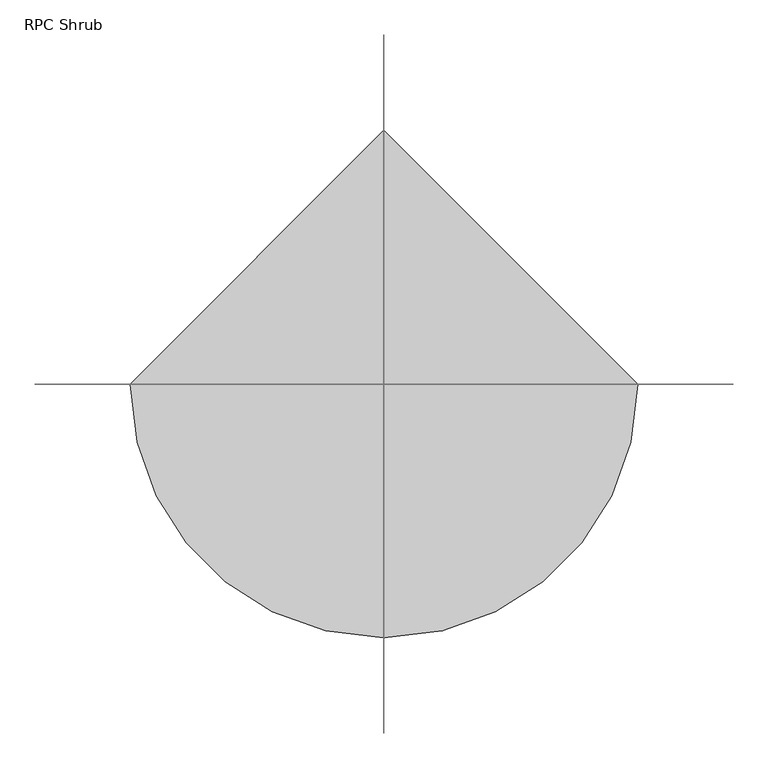
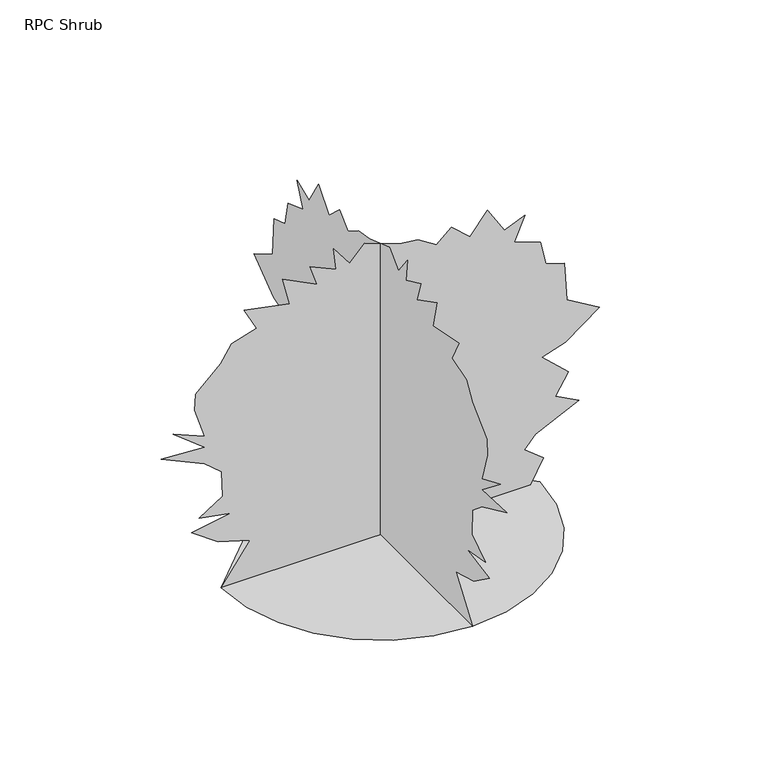
"""IFC4 building model written with IfcOpenShell, lengths in millimetres: geographic element geometry, RPC Shrub."""

from ifc_helpers import new_model, si_unit, origin, place, context, project, spatial, triangles, source, transform, mapped, element, save


def rpc_shrub_d2795376(model_context):
    return source(origin(), model_context, "Body", "Tessellation", [
        triangles([(-812.5409557, 0.0, 3.62e-05), (-791.0601448, -186.180478, 3.62e-05), (-729.8816843, -357.1570149, 3.62e-05), (-633.9078186, -508.0330164, 3.62e-05), (-508.0330164, -633.9078186, 3.62e-05), (-357.1570149, -729.8816843, 3.62e-05), (-186.180478, -791.0601448, 3.62e-05), (3.55e-05, -812.5409557, 3.62e-05), (186.180478, -791.0601448, 3.62e-05), (357.1570149, -729.8816843, 3.62e-05), (508.0330164, -633.9078186, 3.62e-05), (633.9078186, -508.0330164, 3.62e-05), (729.8816843, -357.1570149, 3.62e-05), (791.0601448, -186.180478, 3.62e-05), (812.5409557, 7.1e-05, 3.62e-05), (-0.0001066, 812.5409557, 3.62e-05), (-0.0042747, -811.2988804, 0.0001209), (-0.0042708, -665.7314575, 204.5081021), (-0.004267, -827.9002653, 251.4511125), (-0.004262, -964.4608252, 349.6055863), (-0.004264, -763.884696, 383.7457263), (-0.0042607, -926.0535038, 413.6186849), (-0.0042602, -806.5617422, 490.4333639), (-0.0042562, -810.8289963, 622.7267424), (-0.0042527, -896.1805452, 695.2767471), (-0.0042464, -1118.0927267, 797.697167), (-0.0042501, -896.1805452, 784.8930067), (-0.0042438, -1058.3468822, 912.9192038), (-0.0042483, -896.1805452, 844.6389238), (-0.0042428, -947.3895561, 1002.5380068), (-0.0042404, -943.1223021, 1087.8896284), (-0.0042387, -815.0961777, 1207.38139), (-0.0042368, -759.6175146, 1297.000193), (-0.0042376, -631.5913176, 1335.4075871), (-0.0042331, -695.6044161, 1454.899276), (-0.0042379, -465.1578355, 1407.9550484), (-0.0042331, -499.2979754, 1553.0525871), (-0.0042384, -324.3300579, 1463.4336388), (-0.0042347, -358.4701979, 1570.1213127), (-0.0042384, -226.1755659, 1510.3753956), (-0.0042348, -238.9781819, 1625.6000484), (-0.0042392, -157.8947773, 1518.9123745), (-0.0042379, -81.0790899, 1599.9941986), (-0.0042425, 98.1577894, 1535.9812454), (-0.0042443, 192.0433106, 1523.1795559), (-0.0042475, 285.9303487, 1463.4336388), (-0.0042466, 362.7450096, 1531.7139187), (-0.0042505, 456.6310304, 1446.3622971), (-0.0042486, 546.2498697, 1557.3197685), (-0.0042539, 631.6014914, 1420.7592087), (-0.0042542, 738.2890926, 1463.4336388), (-0.0042571, 682.8104296, 1339.6747684), (-0.0042604, 815.1063515, 1292.7303955), (-0.0042647, 844.9766939, 1164.7042711), (-0.004267, 938.862751, 1134.8313852), (-0.0042731, 951.6669113, 934.2577269), (-0.0042786, 1118.1003571, 836.1044884), (-0.0042798, 943.1324759, 708.078364), (-0.0042791, 823.6407143, 669.67097), (-0.004285, 960.2012741, 541.6448456), (-0.0042871, 891.9209942, 434.9546645), (-0.0042908, 1011.4127558, 370.9416023), (-0.0042907, 789.5005743, 264.2539829), (-0.0042918, 734.0219112, 200.2406482), (-0.0042955, 832.1751497, 123.4246974), (-0.0042982, 766.4170269, 0.0205859), (-811.3090542, 0.0043453, 0.0), (-665.7416313, 0.0043331, 204.5081021), (-827.9078957, 0.0043303, 251.4511125), (-964.4684555, 0.0043245, 349.6055863), (-763.8948698, 0.0043224, 383.7457263), (-926.0611341, 0.0043206, 413.6186849), (-806.5693726, 0.0043161, 490.4333639), (-810.836554, 0.0043082, 622.7267424), (-896.1881756, 0.0043039, 695.2742037), (-1118.1003571, 0.0042978, 797.697167), (-896.1881756, 0.0042985, 784.8930067), (-1058.3545126, 0.0042909, 912.9192038), (-896.1881756, 0.004295, 844.6389238), (-947.3996572, 0.0042855, 1002.5380068), (-943.1299324, 0.0042805, 1087.8896284), (-815.1063515, 0.0042733, 1207.38139), (-759.6276157, 0.004268, 1297.000193), (-631.6014914, 0.0042657, 1335.4075871), (-695.6145899, 0.0042586, 1454.899276), (-465.1654295, 0.0042614, 1407.9550484), (-499.3055695, 0.0042527, 1553.0525871), (-324.3376883, 0.0042581, 1463.4336388), (-358.4778282, 0.0042517, 1570.1213127), (-226.1839592, 0.0042553, 1510.3753956), (-238.9868297, 0.0042484, 1625.6000484), (-157.903425, 0.0042548, 1518.9123745), (-81.0877195, 0.0042499, 1599.9941986), (98.1491599, 0.0042537, 1535.9812454), (192.0346629, 0.0042545, 1523.1795559), (285.9201749, 0.0042581, 1463.4336388), (362.7374156, 0.004254, 1531.7139187), (456.6234364, 0.0042591, 1446.3622971), (546.2422394, 0.0042525, 1557.3197685), (631.5913176, 0.0042606, 1420.7565926), (738.2814623, 0.0042581, 1463.4336388), (682.8027992, 0.0042654, 1339.6747684), (815.0961777, 0.0042682, 1292.7303955), (844.9691362, 0.0042759, 1164.7042711), (938.8551207, 0.0042777, 1134.8313852), (951.6567375, 0.0042896, 934.2577269), (1118.0927267, 0.0042955, 836.1044884), (943.1223021, 0.0043031, 708.078364), (823.6305405, 0.0043054, 669.67097), (960.1936438, 0.004313, 541.6448456), (891.9133638, 0.0043194, 434.9546645), (1011.402582, 0.0043232, 370.9416023), (789.4904005, 0.0043296, 264.2539829), (734.0142809, 0.0043334, 200.2403938), (832.1675194, 0.0043379, 123.4246974), (766.4094692, 0.0043453, 0.020512)], [[15, 16, 1], [14, 15, 1], [14, 1, 2], [13, 14, 2], [13, 2, 3], [13, 3, 4], [12, 13, 4], [11, 12, 4], [11, 4, 5], [11, 5, 6], [11, 6, 7], [11, 7, 8], [11, 8, 9], [11, 9, 10], [27, 28, 29], [25, 26, 27], [40, 41, 42], [21, 22, 23], [50, 51, 52], [19, 20, 21], [38, 39, 40], [36, 37, 38], [34, 35, 36], [61, 62, 63], [66, 17, 18], [56, 57, 58], [48, 49, 50], [18, 19, 21], [46, 47, 48], [64, 65, 66], [59, 60, 61], [56, 58, 59], [54, 55, 56], [42, 43, 44], [52, 53, 54], [54, 56, 59], [24, 25, 27], [48, 50, 52], [59, 61, 63], [52, 54, 59], [48, 52, 59], [46, 48, 59], [66, 18, 21], [30, 31, 32], [29, 30, 32], [66, 21, 23], [66, 23, 24], [64, 66, 24], [63, 64, 24], [59, 63, 24], [46, 59, 24], [45, 46, 24], [44, 45, 24], [42, 44, 24], [40, 42, 24], [38, 40, 24], [36, 38, 24], [34, 36, 24], [34, 24, 27], [34, 27, 29], [34, 29, 32], [33, 34, 32], [77, 78, 79], [75, 76, 77], [90, 91, 92], [71, 72, 73], [100, 101, 102], [69, 70, 71], [88, 89, 90], [86, 87, 88], [84, 85, 86], [111, 112, 113], [116, 67, 68], [106, 107, 108], [98, 99, 100], [68, 69, 71], [96, 97, 98], [114, 115, 116], [109, 110, 111], [106, 108, 109], [104, 105, 106], [92, 93, 94], [102, 103, 104], [104, 106, 109], [74, 75, 77], [98, 100, 102], [109, 111, 113], [102, 104, 109], [98, 102, 109], [96, 98, 109], [116, 68, 71], [80, 81, 82], [79, 80, 82], [116, 71, 73], [116, 73, 74], [114, 116, 74], [113, 114, 74], [109, 113, 74], [96, 109, 74], [95, 96, 74], [94, 95, 74], [92, 94, 74], [90, 92, 74], [88, 90, 74], [86, 88, 74], [84, 86, 74], [84, 74, 77], [84, 77, 79], [84, 79, 82], [83, 84, 82]], closed=False),
    ])


if __name__ == "__main__":
    model = new_model("IFC4")
    model_context = context("Model", 3, world=origin())
    ifc_project = project(units=[si_unit("LENGTHUNIT", "METRE", prefix="MILLI")], contexts=[model_context])
    site = spatial("IfcSite", under=ifc_project)
    building = spatial("IfcBuilding", under=site)
    placement = place(None, origin())
    rpc_shrub_shape = rpc_shrub_d2795376(model_context)
    element("IfcGeographicElement", 1, ObjectType="RPC Shrub", at=placement, inside=building, context=model_context, shape_type="MappedRepresentation", body=[
        mapped(rpc_shrub_shape, transform((0.0, 0.0, 0.0), x_axis=(1.0, 0.0, 0.0), y_axis=(0.0, 1.0, 0.0), z_axis=(0.0, 0.0, 1.0))),
    ])
    save(model, "model.ifc")

# Revit data of these elements
# Type "RPC Shrub"
#   built-in parameter 1005198 = "{2, 15},{39, RPC-16-G3GJ-A6PX-PK1P-U000-ST1L-LVER-AU},{1, 0},{1, 0},{2, 35},{1, 8},{5, Color},{1, 0},{1, 0},{3, 0.8},{3, 0.8},{3, 0.8},{1, 8},{7, BBoxMin},{1, 0},{1, 0},{1, 0},{1, 0},{1, 0},{1, 8},{7, BBoxMax},{1, 0},{1, 0},{1, 0},{1, 0},{1, 0},{2, 11},{9, RPCTypeId},{1, 0},{1, 0},{39, RPC-16-G3GJ-A6PX-PK1P-U000-ST1L-LVER-AU},{1, 6},{14, RPCPlantHeight},{1, 0},{1, 0},{7, 5.33333},{2, 11},{7, keyword},{1, 0},{1, 0},{22, :Geometry:RPC:Oleander},{2, 11},{8, category},{1, 0},{1, 0},{17, :Shrubs & Grasses},{2, 11},{12, LocalizedUID},{1, 0},{1, 0},{8, Oleander},{2, 14},{6, Height},{1, 0},{1, 0},{7, 5.33333},{1, 2},{16, Cast Reflections},{1, 0},{1, 0},{1, 0},{1, 2},{12, Cast Shadows},{1, 0},{1, 0},{1, 1},{1, 2},{9, Lock View},{1, 0},{1, 0},{1, 0},{1, 4},{5, ViewC},{1, 0},{1, 0},{1, 0},{2, 11},{20, AdvancedUIDefinition},{1, 0},{1, 0},{0, },{2, 11},{10, AssetLibID},{1, 0},{1, 0},{36, 4D3F6E72-3F99-4203-98E9-AF80B3C7A7A4},{2, 11},{10, BaseSchema},{1, 0},{1, 0},{9, RPCSchema},{2, 11},{12, ExchangeGUID},{1, 0},{1, 0},{0, },{1, 2},{6, Hidden},{1, 0},{1, 0},{1, 0},{1, 4},{11, RPCCategory},{1, 0},{1, 0},{1, 0},{2, 11},{8, RPCImage},{1, 0},{1, 0},{0, },{1, 4},{13, SchemaVersion},{1, 0},{1, 0},{1, 4},{2, 11},{12, UIDefinition},{1, 0},{1, 0},{0, },{2, 11},{6, UIName},{1, 0},{1, 0},{39, RPC-16-G3GJ-A6PX-PK1P-U000-ST1L-LVER-AU},{2, 11},{11, VersionGUID},{1, 0},{1, 0},{9, RPCSchema},{2, 11},{9, assettype},{1, 0},{1, 0},{11, RPCGeometry},{2, 11},{11, description},{1, 0},{1, 0},{0, },{2, 11},{9, localname},{1, 0},{1, 0},{3, RPC},{2, 11},{9, localtype},{1, 0},{1, 0},{3, RPC},{1, 4},{8, revision},{1, 0},{1, 0},{1, 1},{2, 11},{9, thumbnail},{1, 0},{1, 0},{0, },{1, 4},{7, version},{1, 0},{1, 0},{1, 1},{1, 2},{20, RPC_Cast Reflections},{1, 0},{1, 0},{1, 1},{1, 2},{16, RPC_Cast Shadows},{1, 0},{1, 0},{1, 1},{1, 2},{13, RPC_Lock View},{1, 0},{1, 0},{1, 0},{1, 4},{9, RPC_ViewC},{1, 0},{1, 0},{1, 0},{21, assetlibrary_base.fbx},{1, 5},"
#   built-in parameter 1005195 = "RPC-16-G3GJ-A6PX-PK1P-U000-ST1L-LVER-AU"
#   Assembly Code = "G2050500"
#   Height = 5' - 4"
#   Default Elevation = 0
